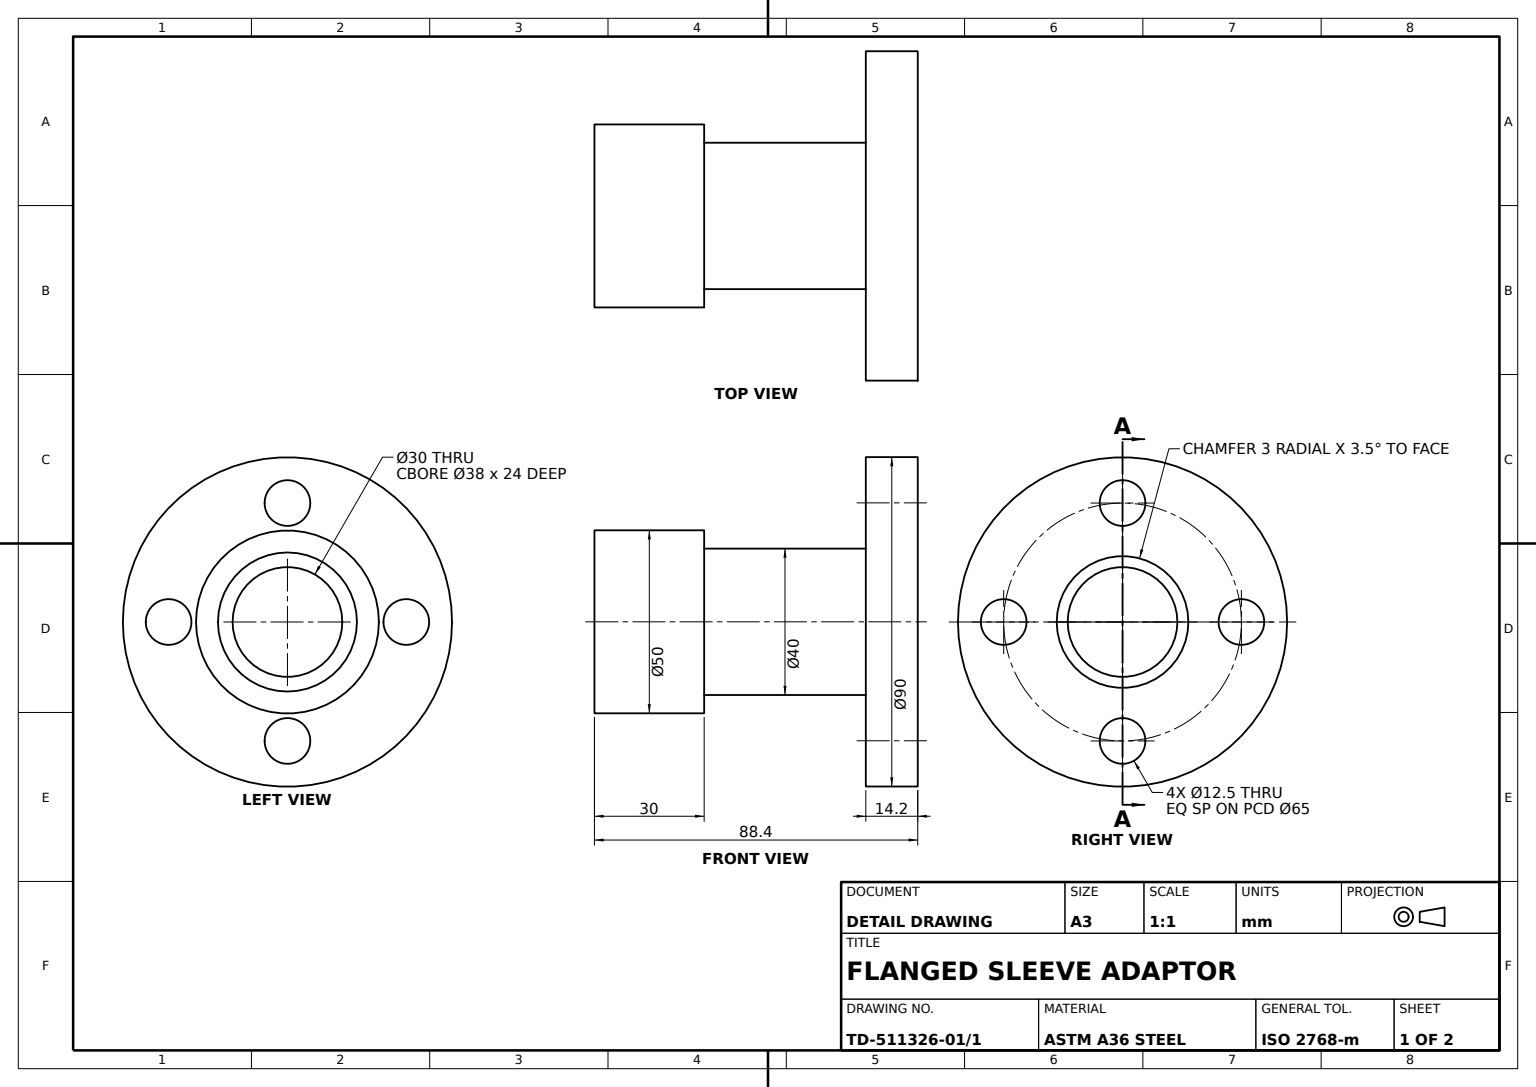
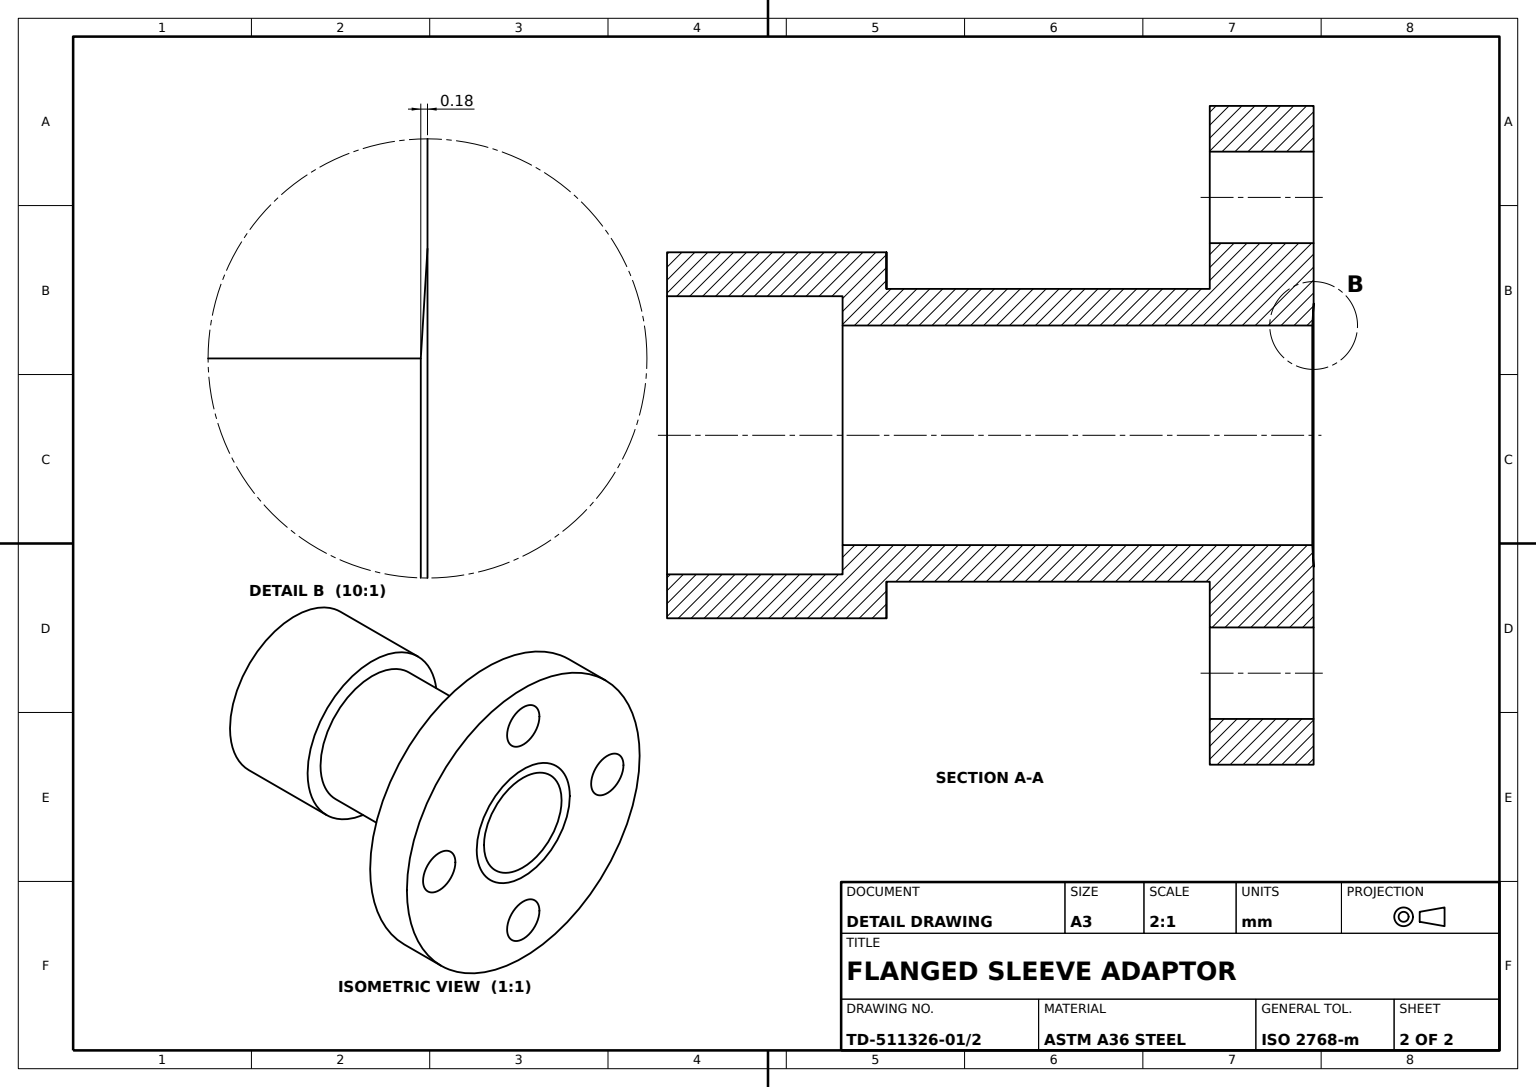
SolidWorks part; units mm, degrees
material "ASTM A36 Steel"
ref_plane "Front Plane" through (0, 0, 0) normal (0, 0, 1) x (1, 0, 0)
ref_plane "Top Plane" through (0, 0, 0) normal (0, 1, 0) x (1, 0, 0)
ref_plane "Right Plane" through (0, 0, 0) normal (1, 0, 0) x (0, 0, -1)
sketch "Sleeve Profile Sketch" plane through (0, 0, 0) normal (0, 0, 1) x (1, 0, 0)
  line L0 (0, 0) -> (0, 45)
  line L1 (0, 45) -> (-14.2, 45)
  line L2 (-14.2, 45) -> (-14.2, 20)
  line L3 (-14.2, 20) -> (-58.4, 20)
  line L4 (-58.4, 20) -> (-58.4, 25)
  line L5 (-58.4, 25) -> (-88.4, 25)
  line L6 (-88.4, 25) -> (-88.4, 0)
  line L7 (-88.4, 0) -> (0, 0)
  dimension "D1" = 30
  dimension "D2" = 44.2
  dimension "D3" = 14.2
  dimension "D4" = 45
  dimension "D5" = 25
  dimension "D6" = 20
revolve "Flanged Sleeve Body" add sketch "Sleeve Profile Sketch" angle 360 about L7
sketch "Bolt Holes Sketch" plane through (-14.2, 0, 0) normal (-1, 0, 0) x (0, 0, 1)
  circle A0 centre (0, 0) radius 32.5 construction
  circle A1 centre (0, -32.5) radius 6.25
  circle A2 centre (-32.5, 0) radius 6.25
  circle A3 centre (0, 32.5) radius 6.25
  circle A4 centre (32.5, 0) radius 6.25
  point P14 (0, 0)
  dimension "D1" = 65
  dimension "D2" = 12.5
  dimension "D3" = 4
extrude "Flange Bolt Holes 4xØ12.5" cut sketch "Bolt Holes Sketch" against normal through all
sketch "Counterbore Sketch" plane through (-88.4, 0, 0) normal (-1, 0, 0) x (0, 0, 1)
  circle A0 centre (0, 0) radius 19
  dimension "D1" = 38
extrude "Counterbore Ø38x24" cut sketch "Counterbore Sketch" against normal blind 24
sketch "Through Bore Sketch" plane through (0, 0, 0) normal (1, 0, 0) x (0, 0, -1)
  circle A0 centre (0, 0) radius 15
  dimension "D1" = 30
extrude "Through Bore Ø30" cut sketch "Through Bore Sketch" against normal up to next
chamfer "Bore Chamfer 3mm" distance 3 angle 3.5 1 edges at (0, 0, -15)
